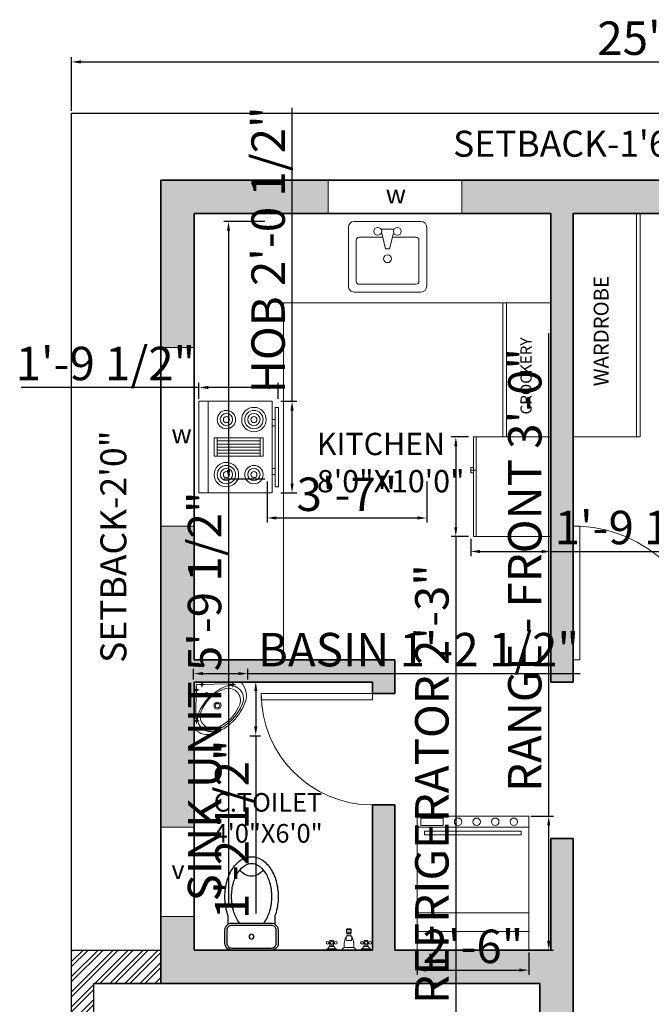
# Model space of a CAD drawing. Units: inches. Extents: x 3488 to 4319, y 780 to 1756.
# Tile 4 of 8: x 3509 to 3679, y 1491 to 1756. Entities that reach past the tile are written whole.
import ezdxf

# ---------------------------------------------------------------- set-up
doc = ezdxf.new("R2010")
doc.units = ezdxf.units.IN
for name, color, linetype, lineweight in [('A-ANNO-IDEN', 7, 'Continuous', 13), ('A-ANNO-TEXT', 7, 'Continuous', 18), ('A-AREA-IDEN', 7, 'Continuous', 18), ('A-DOOR', 4, 'Continuous', 18), ('A-EQPM', 8, 'Continuous', 18), ('A-FLOR-CASE', 32, 'Continuous', 18), ('A-WALL', 7, 'Continuous', 35), ('A-WALL-PATT', 252, 'Continuous', 13), ('C-PROP', 7, 'Continuous', 25), ('DIM', 9, 'Continuous', 18), ('L-FENC', 7, 'Continuous', 30), ('L-FENC-PATT', 251, 'Continuous', 13), ('window', 130, 'Continuous', 18), ('Сантехника', 9, 'Continuous', 18)]:
    doc.layers.add(name, color=color, linetype=linetype, lineweight=lineweight)
doc.layers.add('SANTEH', color=7, linetype='Continuous')
doc.styles.add('ATT', font='romans.shx')
doc.styles.get("Standard").update_dxf_attribs({"font": 'arial.ttf'})
doc.dimstyles.new('ISO-25', dxfattribs={"dimtxt": 9, "dimasz": 2.5, "dimexe": 1.25, "dimexo": 0.625, "dimtad": 1, "dimdec": 1, "dimlunit": 3, "dimtxsty": 'Standard', "dimcen": 2.5, "dimclrd": 1, "dimclre": 1, "dimclrt": 1, "dimadec": 0, "dimazin": 0, "dimtfac": 1, "dimtdec": 1, "dimtmove": 0, "dimatfit": 3, "dimfxl": 1, "dimarcsym": 0})

# ---------------------------------------------------------------- blocks, each defined once
blk = doc.blocks.new('*U3')
for p, q in [((0, 0), (0, -6)), ((36, 0), (36, -6))]:
    blk.add_line(p, q)
blk.add_lwpolyline([(0, 0), (0, 36), (1.75, 36), (1.75, 0)], close=True)
blk.add_arc((0, 0), 36, 0, 90)
blk = doc.blocks.new('*U4')
for p, q in [((-30, 0), (-30, -6)), ((0, 0), (0, -6))]:
    blk.add_line(p, q)
blk.add_lwpolyline([(0, 0), (0, 30), (-1.75, 30), (-1.75, 0)], close=True)
blk.add_arc((0, 0), 30, 90, 180)
blk = doc.blocks.new('*D5')
at = {"layer": 'Defpoints', "color": 0, "transparency": 16777216}
for p in [(3822.99, 1744.35), (3522.99, 1730.55), (3822.99, 1730.55)]:
    blk.add_point(p, dxfattribs=at)
at = {"layer": 'DIM', "color": 0, "lineweight": -2, "transparency": 16777216}
for p, q in [((3522.99, 1731.18), (3522.99, 1745.6)), ((3822.99, 1731.18), (3822.99, 1745.6)), ((3525.49, 1744.35), (3820.49, 1744.35))]:
    blk.add_line(p, q, dxfattribs=at)
at = {"layer": 'DIM', "color": 0, "transparency": 16777216}
for points in [[(3525.49, 1744.77), (3525.49, 1743.94), (3522.99, 1744.35)], [(3820.49, 1744.77), (3820.49, 1743.94), (3822.99, 1744.35)]]:
    blk.add_solid(points, dxfattribs=at)
at = {"layer": 'DIM', "color": 0, "transparency": 16777216, "insert": (3672.99, 1749.57), "char_height": 9, "attachment_point": 5}
blk.add_mtext("25'", dxfattribs=at)
blk = doc.blocks.new('s_11')
at = {"color": 0}
for p, q in [((-2.8, 5.7), (-3.1, 302.9)), ((-2.8, 5.7), (-3.1, 302.9)), ((11.5, 234), (11.4, 270.2)), ((-6.7, 252.1), (29.6, 252.1)), ((10.9, 19.3), (7.9, 238.3)), ((11.7, 31.1), (11.6, 67.3)), ((-6.5, 49.2), (29.8, 49.2)), ((237.1, 9.4), (18, 12.2)), ((29.8, 13), (66, 13)), ((47.9, -5.2), (47.9, 31.1)), ((232.7, 13), (268.9, 13)), ((250.8, -5.2), (250.8, 31.1)), ((301.6, -1.5), (4.5, -1.5)), ((301.6, -1.5), (4.5, -1.5))]:
    blk.add_line(p, q, dxfattribs=at)
at = {"color": 0, "extrusion": (0, 0, -1)}
for centre, major_axis, start_param, end_param in [((84.1, 218.8), (-87.2, 87.1), 0.025883, 1.117399), ((84.1, 218.8), (-87.2, 87.1), 0.025883, 1.117399), ((105.4, 236.4), (-61.5, 61.5), -1.180146, 1.180146), ((14.2, 15.4), (-239.5, 239.2), 1.117399, 2.024193), ((14.2, 15.4), (-239.5, 239.2), 1.117399, 2.024193), ((4.2, 302.9), (-5.13, 5.12), -0.785398, 0.025884), ((4.2, 302.9), (-5.13, 5.12), -0.785398, 0.025884), ((11.5, 252.1), (-5.13, 5.12), 3.141593, 9.424778), ((116.1, 223.2), (-56.4, 56.4), -1.140724, 1.140724), ((13.2, 14.4), (-231.7, 231.5), 1.180146, 1.961447), ((54, 55.3), (-183.1, 183), 1.140724, 2.000869), ((327.3, 328.9), (-231.7, 231.5), 4.321738, 5.10304), ((283.9, 285.4), (-183.1, 183), 4.282316, 5.142462), ((150.8, 152.2), (-16.4, 16.4), 3.141593, 9.424778), ((150.8, 152.2), (-10.3, 10.2), 3.141593, 9.424778), ((221.8, 117.6), (-56.4, 56.4), 2.000869, 4.282316), ((235, 106.9), (-61.5, 61.5), 1.961447, 4.321738), ((79.1, 80.4), (-8.98, 8.97), 3.141593, 9.424778), ((217.5, 85.5), (-87.2, 87.1), 2.024193, 3.11571), ((217.5, 85.5), (-87.2, 87.1), 2.024193, 3.11571), ((4.5, 5.7), (-5.13, 5.12), 3.926991, 5.497787), ((4.5, 5.7), (-5.13, 5.12), 3.926991, 5.497787), ((11.7, 49.2), (-5.13, 5.12), 3.141593, 9.424778), ((18.1, 19.4), (-5.13, 5.12), 3.939487, 5.485291), ((47.9, 13), (-5.13, 5.12), 3.141593, 9.424778), ((250.8, 13), (-5.13, 5.12), 3.141593, 9.424778), ((301.6, 5.7), (-5.13, 5.12), 3.115708, 3.926991), ((301.6, 5.7), (-5.13, 5.12), 3.115708, 3.926991)]:
    blk.add_ellipse(centre, major_axis=major_axis, ratio=0.999043, start_param=start_param, end_param=end_param, dxfattribs=at)
blk = doc.blocks.new('K10-44')
at = {"layer": 'SANTEH'}
for points in [[(-182, 222.6, 0.020439), (-174, 197.6), (-174, 134.8, 0.262987), (-198.2, 92), (-198.2, -8, 0.414214), (-148.2, -58), (151.8, -58, 0.414214), (201.8, -8), (201.8, 92, 0.262987), (177.6, 134.8), (177.6, 197.6, 0.020439), (185.6, 222.6, 0.067459), (201.8, 342, 0.067459), (185.6, 461.3, 0.079812), (143.2, 554.1, 0.107118), (73.7, 621.5, 0.139889), (1.8, 642, 0.139889), (-70.1, 621.5, 0.107118), (-139.6, 554.1, 0.079812), (-182, 461.3, 0.067459), (-198.2, 342, 0.067459)], [(-148.2, 127), (151.8, 127, -0.414214), (186.8, 92), (186.8, -8, -0.414214), (151.8, -43), (-148.2, -43, -0.414214), (-183.2, -8), (-183.2, 92, -0.414214)]]:
    blk.add_lwpolyline(points, format="xyb", close=True, dxfattribs=at)
for points in [[(89.9, 142, 0.027307), (101.6, 157.6, 0.079812), (137.4, 235.9, 0.067459), (151.8, 342, 0.067459), (137.4, 448, 0.079812), (101.6, 526.4, 0.107118), (47.3, 579, 0.139889), (1.8, 592, 0.139889), (-43.7, 579, 0.107118), (-98, 526.4, 0.079812), (-133.8, 448, 0.067459), (-148.2, 342, 0.067459), (-133.8, 235.9, 0.079812), (-98, 157.6, 0.027307), (-86.4, 142, 0.139889)], [(-174, 134.8, -0.136371), (-148.2, 142), (151.8, 142, -0.136371), (177.6, 134.8)]]:
    blk.add_lwpolyline(points, format="xyb", dxfattribs=at)
blk.add_circle((1.8, 42), 18.3, dxfattribs=at)
blk.add_arc((1.8, 601.6), 105.3, 213.89944, 326.10056, dxfattribs=at)
blk = doc.blocks.new('Faucet - Bathroom front')
for p, q in [((-0.5, 4.25), (0.5, 4.25)), ((0.5, 3.75), (-0.5, 3.75)), ((-0.5, 3), (0.5, 3)), ((-0.25, 3), (-0.25, 3.5)), ((0.25, 3.5), (0.25, 3)), ((-5, 0), (-2.25, 0)), ((-4.5087, 0.25), (-2.7408, 0.25)), ((-4, 1.625), (-4.25, 1.625)), ((-4, 1.375), (-4.25, 1.375)), ((-3.1442, 0.75), (-4.0979, 0.75)), ((-3.25, 1.625), (-3, 1.625)), ((-3.25, 1.375), (-3, 1.375)), ((-1.5, 0), (1.5, 0)), ((-1, 0.5), (1, 0.5)), ((0.5, 2), (-0.5, 2)), ((2.25, 0), (5, 0)), ((2.7413, 0.25), (4.5092, 0.25)), ((3.25, 1.625), (3, 1.625)), ((3.25, 1.375), (3, 1.375)), ((4.1058, 0.75), (3.1521, 0.75)), ((4, 1.625), (4.25, 1.625)), ((4, 1.375), (4.25, 1.375))]:
    blk.add_line(p, q)
for points in [[(-0.5, 3.75), (-0.5, 4.25)], [(-0.25, 4.5), (0.25, 4.5)], [(0.5, 4.25), (0.5, 3.75)], [(0.25, 3.5), (-0.25, 3.5)]]:
    blk.add_lwpolyline(points)
for points in [[(-4, 1), (-4, 2), (-3.25, 2), (-3.25, 1)], [(3.25, 1), (3.25, 2), (4, 2), (4, 1)]]:
    blk.add_lwpolyline(points, close=True)
for centre in [(-4.5, 1.5), (-3.625, 1.5), (-2.75, 1.5), (2.75, 1.5), (3.625, 1.5), (4.5, 1.5)]:
    blk.add_circle(centre, 0.2795)
for centre, radius, start, end in [((-0.2575, 4.2575), 0.2426, 88.22243, 181.7776), ((0.2575, 4.2575), 0.2426, 358.2224, 91.77757), ((3, 1), 4.0311, 150.2551, 187.125), ((0.6413, 2.5), 1.246, 156.3417, 203.6583), ((-0.2575, 3.7425), 0.2426, 178.2224, 271.7776), ((0.2575, 3.7425), 0.2426, 268.2224, 1.777565), ((-3, 1), 4.0311, 352.875, 29.74488), ((-0.6413, 2.5), 1.246, 336.3417, 23.65835), ((-5.375, 1.375), 1.4252, 285.2551, 344.7449), ((-1.875, 1.375), 1.4252, 195.2551, 254.7449), ((-0.7962, -0.2038), 0.7327, 106.1502, 163.8498), ((0.7962, -0.2038), 0.7327, 16.1502, 73.84979), ((1.875, 1.375), 1.4252, 285.2551, 344.7449), ((5.375, 1.375), 1.4252, 195.2551, 254.7449)]:
    blk.add_arc(centre, radius, start, end)
blk = doc.blocks.new('Range-Oven - 30 in top')
for p, q in [((0, -3), (30, -3)), ((12, -6), (18, -6)), ((13, -20), (13, -6)), ((14, -6), (14, -20)), ((15, -20), (15, -6)), ((16, -6), (16, -20)), ((17, -20), (17, -6)), ((18, -20), (12, -20)), ((6, -24), (6, -25)), ((8, -25), (8, -24)), ((22, -25), (22, -24)), ((24, -24), (24, -25))]:
    blk.add_line(p, q)
for points in [[(0, -24), (0, 0), (30, 0), (30, -24)], [(12, -21), (12, -5), (18, -5), (18, -21)], [(2, -26), (2, -25), (28, -25), (28, -26)]]:
    blk.add_lwpolyline(points, close=True)
for centre, radius in [((6, -9), 4), ((6, -9), 3), ((24, -9), 3), ((6, -9), 2), ((6, -9), 1), ((24, -9), 2), ((24, -9), 1), ((6, -18), 3), ((6, -18), 2), ((24, -18), 4), ((24, -18), 3), ((24, -18), 2), ((6, -18), 1), ((24, -18), 1)]:
    blk.add_circle(centre, radius)
blk = doc.blocks.new('Range-Oven - 30 in front')
for p, q in [((0, 33.00005), (30, 33.00005)), ((30, 10), (0, 10)), ((0, 5), (30, 5))]:
    blk.add_line(p, q)
for points in [[(0, 0), (0, 36.00005), (30, 36.00005), (30, 0)], [(1, 33.50005), (1, 35.50005), (7, 35.50005), (7, 33.50005)], [(2, 31.00005), (2, 32.00005), (28, 32.00005), (28, 31.00005)]]:
    blk.add_lwpolyline(points, close=True)
for centre in [(11, 34.50005), (16, 34.50005), (21, 34.50005), (26, 34.50005)]:
    blk.add_circle(centre, 1)
blk = doc.blocks.new('Refrigerator-2 door - 36 in top')
for p, q in [((0, -26.999999), (36, -26.999999)), ((11, -27.999999), (11, -28.999999)), ((12, -26.999999), (12, -28.999999)), ((13, -28.999999), (13, -27.999999)), ((11, -28.999999), (13, -28.999999))]:
    blk.add_line(p, q)
blk.add_lwpolyline([(0, -27.999999), (0, 0), (36, 0), (36, -27.999999)], close=True)
blk = doc.blocks.new('15PLAV06')
at = {"color": 0, "linetype": 'ByBlock'}
for p, q in [((0, 8.5), (0, -8.5)), ((16.5, 10), (1.5, 10)), ((4.75, 8), (15.25, 8)), ((18, -8.5), (18, 8.5)), ((4, 1.25), (4, 7.25)), ((16, 7.25), (16, -7.25)), ((2, -1.5), (2, 1.5)), ((7, 0.5), (3, 1.5)), ((7, -0.5), (7, 0.5)), ((3, -1.5), (7, -0.5)), ((4, -7.25), (4, -1.25)), ((1.5, -10), (16.5, -10)), ((15.25, -8), (4.75, -8))]:
    blk.add_line(p, q, dxfattribs=at)
for centre in [(2.5, 2.5), (9.5, 0), (2.5, -2.5)]:
    blk.add_circle(centre, 1, dxfattribs=at)
for centre, radius, start, end in [((1.5, 8.5), 1.5, 90, 180), ((4.75, 7.25), 0.75, 90, 180), ((15.25, 7.25), 0.75, 0, 90), ((16.5, 8.5), 1.5, 0, 90), ((4.75, -7.25), 0.75, 180, 270), ((15.25, -7.25), 0.75, 270, 0), ((1.5, -8.5), 1.5, 180, 270), ((16.5, -8.5), 1.5, 270, 0)]:
    blk.add_arc(centre, radius, start, end, dxfattribs=at)
at = {"color": 0, "linetype": 'ByBlock', "style": 'ATT'}
for tag, p, flags in [('ITEM', (0, -20), 3), ('ROOM_NUMBER', (0, -29), 1)]:
    blk.add_attdef(tag, p, '', height=6, dxfattribs=dict(at, flags=flags))
blk = doc.blocks.new('*D84')
at = {"layer": 'Defpoints', "color": 0, "transparency": 16777216}
for p in [(3570.37, 1579.88), (3555.83, 1577.7), (3570.37, 1577.7)]:
    blk.add_point(p, dxfattribs=at)
at = {"layer": 'DIM', "color": 1, "lineweight": -2, "transparency": 16777216}
for p, q in [((3555.83, 1578.33), (3555.83, 1581.13)), ((3570.37, 1578.33), (3570.37, 1581.13)), ((3558.33, 1579.88), (3567.87, 1579.88)), ((3570.37, 1579.88), (3659.84, 1579.88))]:
    blk.add_line(p, q, dxfattribs=at)
at = {"layer": 'DIM', "color": 1, "transparency": 16777216}
for points in [[(3558.33, 1580.3), (3558.33, 1579.46), (3555.83, 1579.88)], [(3567.87, 1580.3), (3567.87, 1579.46), (3570.37, 1579.88)]]:
    blk.add_solid(points, dxfattribs=at)
at = {"layer": 'DIM', "color": 1, "transparency": 16777216, "insert": (3616.35, 1585.16), "char_height": 9, "attachment_point": 5}
blk.add_mtext('BASIN 1\'-2 1/2"', dxfattribs=at)
blk = doc.blocks.new('*D85')
at = {"layer": 'Defpoints', "color": 0, "transparency": 16777216}
for p in [(3570.37, 1577.7), (3570.37, 1563.17), (3572.55, 1563.17)]:
    blk.add_point(p, dxfattribs=at)
at = {"layer": 'DIM', "color": 1, "lineweight": -2, "transparency": 16777216}
for p, q in [((3570.99, 1577.7), (3573.8, 1577.7)), ((3572.55, 1575.2), (3572.55, 1565.67)), ((3570.99, 1563.17), (3573.8, 1563.17)), ((3572.55, 1563.17), (3572.55, 1515.37))]:
    blk.add_line(p, q, dxfattribs=at)
at = {"layer": 'DIM', "color": 1, "transparency": 16777216}
for points in [[(3572.13, 1575.2), (3572.96, 1575.2), (3572.55, 1577.7)], [(3572.13, 1565.67), (3572.96, 1565.67), (3572.55, 1563.17)]]:
    blk.add_solid(points, dxfattribs=at)
at = {"layer": 'DIM', "color": 1, "transparency": 16777216, "insert": (3567.27, 1538.02), "char_height": 9, "attachment_point": 5, "rotation": 90}
blk.add_mtext('1\'-2 1/2"', dxfattribs=at)
blk = doc.blocks.new('*D86')
at = {"layer": 'Defpoints', "color": 0, "transparency": 16777216}
for p in [(3578.62, 1653.11), (3582.32, 1653.11), (3578.62, 1628.45)]:
    blk.add_point(p, dxfattribs=at)
at = {"layer": 'DIM', "color": 1, "lineweight": -2, "transparency": 16777216}
for p, q in [((3582.32, 1653.11), (3582.32, 1732.01)), ((3579.25, 1653.11), (3583.57, 1653.11)), ((3582.32, 1630.95), (3582.32, 1650.61)), ((3579.25, 1628.45), (3583.57, 1628.45))]:
    blk.add_line(p, q, dxfattribs=at)
at = {"layer": 'DIM', "color": 1, "transparency": 16777216}
for points in [[(3581.9, 1650.61), (3582.74, 1650.61), (3582.32, 1653.11)], [(3581.9, 1630.95), (3582.74, 1630.95), (3582.32, 1628.45)]]:
    blk.add_solid(points, dxfattribs=at)
at = {"layer": 'DIM', "color": 1, "transparency": 16777216, "insert": (3577.04, 1693.81), "char_height": 9, "attachment_point": 5, "rotation": 90}
blk.add_mtext('HOB 2\'-0 1/2"', dxfattribs=at)
blk = doc.blocks.new('*D87')
at = {"layer": 'Defpoints', "color": 0, "transparency": 16777216}
for p in [(3557.25, 1656.81), (3557.25, 1653.11), (3578.62, 1653.11)]:
    blk.add_point(p, dxfattribs=at)
at = {"layer": 'DIM', "color": 1, "lineweight": -2, "transparency": 16777216}
for p, q in [((3557.25, 1653.74), (3557.25, 1658.06)), ((3578.62, 1653.74), (3578.62, 1658.06)), ((3557.25, 1656.81), (3509.45, 1656.81)), ((3576.12, 1656.81), (3559.75, 1656.81))]:
    blk.add_line(p, q, dxfattribs=at)
at = {"layer": 'DIM', "color": 1, "transparency": 16777216}
for points in [[(3559.75, 1657.23), (3559.75, 1656.39), (3557.25, 1656.81)], [(3576.12, 1657.23), (3576.12, 1656.39), (3578.62, 1656.81)]]:
    blk.add_solid(points, dxfattribs=at)
at = {"layer": 'DIM', "color": 1, "transparency": 16777216, "insert": (3532.1, 1662.09), "char_height": 9, "attachment_point": 5}
blk.add_mtext('1\'-9 1/2"', dxfattribs=at)
blk = doc.blocks.new('*D88')
at = {"layer": 'Defpoints', "color": 0, "transparency": 16777216}
for p in [(3645.99, 1541.55), (3651.39, 1541.55), (3645.99, 1505.55)]:
    blk.add_point(p, dxfattribs=at)
at = {"layer": 'DIM', "color": 1, "lineweight": -2, "transparency": 16777216}
for p, q in [((3651.39, 1541.55), (3651.39, 1671.44)), ((3646.61, 1541.55), (3652.64, 1541.55)), ((3651.39, 1508.05), (3651.39, 1539.05)), ((3646.61, 1505.55), (3652.64, 1505.55))]:
    blk.add_line(p, q, dxfattribs=at)
at = {"layer": 'DIM', "color": 1, "transparency": 16777216}
for points in [[(3650.97, 1539.05), (3651.81, 1539.05), (3651.39, 1541.55)], [(3650.97, 1508.05), (3651.81, 1508.05), (3651.39, 1505.55)]]:
    blk.add_solid(points, dxfattribs=at)
at = {"layer": 'DIM', "color": 1, "transparency": 16777216, "insert": (3646.1, 1607.75), "char_height": 9, "attachment_point": 5, "rotation": 90}
blk.add_mtext('RANGE - FRONT 3\'-0"', dxfattribs=at)
blk = doc.blocks.new('*D89')
at = {"layer": 'Defpoints', "color": 0, "transparency": 16777216}
for p in [(3615.99, 1505.55), (3645.99, 1505.55), (3645.99, 1500.15)]:
    blk.add_point(p, dxfattribs=at)
at = {"layer": 'DIM', "color": 1, "lineweight": -2, "transparency": 16777216}
for p, q in [((3615.99, 1504.93), (3615.99, 1498.9)), ((3645.99, 1504.93), (3645.99, 1498.9)), ((3618.49, 1500.15), (3643.49, 1500.15))]:
    blk.add_line(p, q, dxfattribs=at)
at = {"layer": 'DIM', "color": 1, "transparency": 16777216}
for points in [[(3618.49, 1500.57), (3618.49, 1499.74), (3615.99, 1500.15)], [(3643.49, 1500.57), (3643.49, 1499.74), (3645.99, 1500.15)]]:
    blk.add_solid(points, dxfattribs=at)
at = {"layer": 'DIM', "color": 1, "transparency": 16777216, "insert": (3630.99, 1505.37), "char_height": 9, "attachment_point": 5}
blk.add_mtext('2\'-6"', dxfattribs=at)
blk = doc.blocks.new('*D90')
at = {"layer": 'Defpoints', "color": 0, "transparency": 16777216}
for p in [(3630.4, 1643.52), (3626.38, 1616.73), (3630.4, 1616.73)]:
    blk.add_point(p, dxfattribs=at)
at = {"layer": 'DIM', "color": 1, "lineweight": -2, "transparency": 16777216}
for p, q in [((3629.78, 1643.52), (3625.13, 1643.52)), ((3626.38, 1641.02), (3626.38, 1619.23)), ((3629.78, 1616.73), (3625.13, 1616.73)), ((3626.38, 1616.73), (3626.38, 1486.14))]:
    blk.add_line(p, q, dxfattribs=at)
at = {"layer": 'DIM', "color": 1, "transparency": 16777216}
for points in [[(3625.97, 1641.02), (3626.8, 1641.02), (3626.38, 1643.52)], [(3625.97, 1619.23), (3626.8, 1619.23), (3626.38, 1616.73)]]:
    blk.add_solid(points, dxfattribs=at)
at = {"layer": 'DIM', "color": 1, "transparency": 16777216, "insert": (3621.1, 1550.18), "char_height": 9, "attachment_point": 5, "rotation": 90}
blk.add_mtext('REFRIGERATOR 2\'-3"', dxfattribs=at)
blk = doc.blocks.new('*D91')
at = {"layer": 'Defpoints', "color": 0, "transparency": 16777216}
for p in [(3630.4, 1616.73), (3651.99, 1616.73), (3651.99, 1612.71)]:
    blk.add_point(p, dxfattribs=at)
at = {"layer": 'DIM', "color": 1, "lineweight": -2, "transparency": 16777216}
for p, q in [((3630.4, 1616.1), (3630.4, 1611.46)), ((3651.99, 1616.1), (3651.99, 1611.46)), ((3632.9, 1612.71), (3649.49, 1612.71)), ((3651.99, 1612.71), (3699.79, 1612.71))]:
    blk.add_line(p, q, dxfattribs=at)
at = {"layer": 'DIM', "color": 1, "transparency": 16777216}
for points in [[(3632.9, 1613.13), (3632.9, 1612.29), (3630.4, 1612.71)], [(3649.49, 1613.13), (3649.49, 1612.29), (3651.99, 1612.71)]]:
    blk.add_solid(points, dxfattribs=at)
at = {"layer": 'DIM', "color": 1, "transparency": 16777216, "insert": (3677.14, 1617.99), "char_height": 9, "attachment_point": 5}
blk.add_mtext('1\'-9 1/2"', dxfattribs=at)
blk = doc.blocks.new('*D92')
at = {"layer": 'Defpoints', "color": 0, "transparency": 16777216}
for p in [(3575.62, 1701.45), (3565.22, 1632.12), (3575.62, 1632.12)]:
    blk.add_point(p, dxfattribs=at)
at = {"layer": 'DIM', "color": 1, "lineweight": -2, "transparency": 16777216}
for p, q in [((3575, 1701.45), (3563.97, 1701.45)), ((3565.22, 1698.95), (3565.22, 1634.62)), ((3575, 1632.12), (3563.97, 1632.12)), ((3565.22, 1632.12), (3565.22, 1517.85))]:
    blk.add_line(p, q, dxfattribs=at)
at = {"layer": 'DIM', "color": 1, "transparency": 16777216}
for points in [[(3564.8, 1698.95), (3565.64, 1698.95), (3565.22, 1701.45)], [(3564.8, 1634.62), (3565.64, 1634.62), (3565.22, 1632.12)]]:
    blk.add_solid(points, dxfattribs=at)
at = {"layer": 'DIM', "color": 1, "transparency": 16777216, "insert": (3559.94, 1573.74), "char_height": 9, "attachment_point": 5, "rotation": 90}
blk.add_mtext('SINK UNIT 5\'-9 1/2"', dxfattribs=at)
blk = doc.blocks.new('*D93')
at = {"layer": 'Defpoints', "color": 0, "transparency": 16777216}
for p in [(3575.62, 1632.12), (3618.56, 1632.12), (3618.56, 1621.72)]:
    blk.add_point(p, dxfattribs=at)
at = {"layer": 'DIM', "color": 1, "lineweight": -2, "transparency": 16777216}
for p, q in [((3575.62, 1631.5), (3575.62, 1620.47)), ((3618.56, 1631.5), (3618.56, 1620.47)), ((3578.12, 1621.72), (3616.06, 1621.72))]:
    blk.add_line(p, q, dxfattribs=at)
at = {"layer": 'DIM', "color": 1, "transparency": 16777216}
for points in [[(3578.12, 1622.14), (3578.12, 1621.3), (3575.62, 1621.72)], [(3616.06, 1622.14), (3616.06, 1621.3), (3618.56, 1621.72)]]:
    blk.add_solid(points, dxfattribs=at)
at = {"layer": 'DIM', "color": 1, "transparency": 16777216, "insert": (3597.09, 1626.94), "char_height": 9, "attachment_point": 5}
blk.add_mtext('3\'-7"', dxfattribs=at)

msp = doc.modelspace()

# ---------------------------------------------------------------- hatches: boundary and pattern name
at = {"layer": 'A-WALL-PATT', "transparency": 33554687}
h = msp.add_hatch(color=256, dxfattribs=at)
h.dxf.hatch_style = 1
h.paths.add_polyline_path([(3657.99, 1505.55), (3657.99, 1535.55), (3651.99, 1535.55), (3651.99, 1505.55), (3609.99, 1505.55), (3609.99, 1544.55), (3603.99, 1544.55), (3603.99, 1505.55), (3555.99, 1505.55), (3555.99, 1514.55), (3546.99, 1514.55), (3546.99, 1496.55), (3648.99, 1496.55), (3648.99, 1352.55), (3663.99, 1352.55), (3663.99, 1361.55), (3657.99, 1361.55)])
h.paths.add_polyline_path([(3722.99, 1361.55), (3719, 1361.55), (3703.99, 1361.55), (3703.99, 1352.55), (3722.99, 1352.55)])
h.paths.add_polyline_path([(3798.99, 1397.55), (3789.99, 1397.55), (3789.99, 1361.95), (3789.99, 1361.55), (3770.99, 1361.55), (3770.99, 1352.55), (3798.99, 1352.55)])
h.paths.add_polyline_path([(3798.99, 1547.58), (3789.99, 1547.58), (3789.99, 1463.55), (3798.99, 1463.55)])
h.paths.add_polyline_path([(3798.99, 1613.55), (3789.99, 1613.55), (3789.99, 1583.55), (3693.99, 1583.55), (3693.99, 1577.55), (3789.99, 1577.55), (3789.99, 1571.58), (3798.99, 1571.58)])
h.paths.add_polyline_path([(3798.99, 1712.55), (3717.99, 1712.55), (3717.99, 1703.55), (3789.99, 1703.55), (3789.99, 1673.55), (3798.99, 1673.55)])
h.paths.add_polyline_path([(3681.99, 1712.55), (3627.99, 1712.55), (3627.99, 1703.55), (3651.99, 1703.55), (3651.99, 1577.55), (3657.99, 1577.55), (3657.99, 1703.55), (3681.99, 1703.55)])
h.paths.add_polyline_path([(3591.99, 1712.55), (3546.99, 1712.55), (3546.99, 1667.55), (3555.99, 1667.55), (3555.99, 1703.55), (3591.99, 1703.55)])
edge = h.paths.add_edge_path()
edge.add_line((3555.99, 1619.55), (3546.99, 1619.55))
edge.add_line((3546.99, 1619.55), (3546.99, 1538.55))
edge.add_line((3546.99, 1538.55), (3555.99, 1538.55))
edge.add_line((3555.99, 1538.55), (3555.99, 1565.03))
edge.add_ellipse((3556.27, 1565.11), major_axis=(0.21, 0.21), ratio=0.999043, start_angle=135, end_angle=151.1563, ccw=False)
edge.add_line((3555.98, 1565.08), (3555.99, 1577.26))
edge.add_line((3555.99, 1577.26), (3555.99, 1577.55))
edge.add_line((3555.99, 1577.55), (3603.99, 1577.55))
edge.add_line((3603.99, 1577.55), (3603.99, 1574.55))
edge.add_line((3603.99, 1574.55), (3609.99, 1574.55))
edge.add_line((3609.99, 1574.55), (3609.99, 1583.55))
edge.add_line((3609.99, 1583.55), (3555.99, 1583.55))
edge.add_line((3555.99, 1583.55), (3555.99, 1619.55))
at = {"layer": 'L-FENC-PATT', "transparency": 33554687}
h = msp.add_hatch(dxfattribs=at)
h.set_pattern_fill('ANSI32', color=256, scale=0.3)
h.paths.add_polyline_path([(3546.99, 1505.55), (3522.99, 1505.55), (3522.99, 1310.55), (3546.99, 1310.55), (3546.99, 1316.55), (3528.99, 1316.55), (3528.99, 1496.55), (3546.99, 1496.55)])
h.paths.add_polyline_path([(3756.99, 1316.55), (3642.99, 1316.55), (3642.99, 1310.55), (3756.99, 1310.55)])
h.paths.add_polyline_path([(3822.99, 1316.55), (3792.99, 1316.55), (3792.99, 1310.55), (3822.99, 1310.55)])

# ---------------------------------------------------------------- linework, layer by layer
at = {"layer": 'A-FLOR-CASE'}
for p, q in [((3674.99, 1703.55), (3674.99, 1643.55)), ((3675.99, 1703.55), (3675.99, 1643.55)), ((3579.99, 1679.55), (3651.99, 1679.55)), ((3579.99, 1583.55), (3579.99, 1679.55)), ((3638.99, 1679.55), (3638.99, 1643.52)), ((3639.99, 1679.55), (3639.99, 1643.52)), ((3657.99, 1643.55), (3675.99, 1643.55))]:
    msp.add_line(p, q, dxfattribs=at)
at = {"layer": 'A-WALL'}
for p, q in [((3546.99, 1712.55), (3798.99, 1712.55)), ((3546.99, 1496.55), (3546.99, 1712.55)), ((3555.99, 1703.55), (3651.99, 1703.55)), ((3555.99, 1583.55), (3555.99, 1703.55)), ((3651.99, 1703.55), (3651.99, 1577.55)), ((3657.99, 1703.55), (3657.99, 1577.55)), ((3657.99, 1703.55), (3789.99, 1703.55)), ((3555.99, 1583.55), (3609.99, 1583.55)), ((3609.99, 1574.55), (3609.99, 1583.55)), ((3555.99, 1505.55), (3555.99, 1577.55)), ((3555.99, 1577.55), (3603.99, 1577.55)), ((3603.99, 1574.55), (3603.99, 1577.55)), ((3651.99, 1577.55), (3657.99, 1577.55)), ((3603.99, 1574.55), (3609.99, 1574.55)), ((3603.99, 1505.55), (3603.99, 1544.55)), ((3603.99, 1544.55), (3609.99, 1544.55)), ((3609.99, 1505.55), (3609.99, 1544.55)), ((3651.99, 1535.55), (3657.99, 1535.55)), ((3651.99, 1535.55), (3651.99, 1505.55)), ((3657.99, 1535.55), (3657.99, 1505.55)), ((3555.99, 1505.55), (3603.99, 1505.55)), ((3609.99, 1505.55), (3651.99, 1505.55)), ((3657.99, 1505.55), (3657.99, 1361.55)), ((3528.99, 1496.55), (3648.99, 1496.55)), ((3648.99, 1496.55), (3648.99, 1352.55))]:
    msp.add_line(p, q, dxfattribs=at)
at = {"layer": 'C-PROP'}
for p, q in [((3522.99, 1730.55), (3822.99, 1730.55)), ((3522.99, 1310.55), (3522.99, 1730.55))]:
    msp.add_line(p, q, dxfattribs=at)
at = {"layer": 'L-FENC'}
for p, q in [((3522.99, 1505.55), (3546.99, 1505.55)), ((3528.99, 1316.55), (3528.99, 1496.55))]:
    msp.add_line(p, q, dxfattribs=at)
at = {"layer": 'window'}
for p, q in [((3591.99, 1703.55), (3591.99, 1712.55)), ((3627.99, 1703.55), (3627.99, 1712.55)), ((3555.99, 1667.55), (3546.99, 1667.55)), ((3555.99, 1619.55), (3546.99, 1619.55)), ((3546.99, 1538.55), (3555.99, 1538.55)), ((3546.99, 1514.55), (3555.99, 1514.55))]:
    msp.add_line(p, q, dxfattribs=at)

# ---------------------------------------------------------------- block references
at = {"layer": 'A-DOOR'}
msp.add_blockref('*U3', (3657.99, 1583.55), dxfattribs=at)
at = {"layer": 'A-DOOR', "rotation": 90}
msp.add_blockref('*U4', (3603.99, 1574.55), dxfattribs=at)
at = {"layer": 'A-EQPM'}
for name, p, xscale, yscale, zscale, rotation in [('Range-Oven - 30 in top', (3557.25, 1628.45), 0.8221221388671134, 0.8221221388671134, 0.8221221388671134, 90), ('Refrigerator-2 door - 36 in top', (3651.99, 1643.52), 0.7443170329711898, 0.7443170329711898, 0.7443170329711898, 270)]:
    msp.add_blockref(name, p, dxfattribs=dict(at, xscale=xscale, yscale=yscale, zscale=zscale, rotation=rotation))
msp.add_blockref('Range-Oven - 30 in front', (3615.99, 1505.55), dxfattribs=at)
at = {"layer": 'Сантехника'}
for name, p, xscale, yscale, zscale, rotation in [('15PLAV06', (3608.01, 1701.45), 1.054623354967256, 1.054623354967256, 1.054623354967256, 270), ('s_11', (3556.1, 1577.49), -0.0408764858577606, 0.0408764858577606, 0.0408764858577606, 180)]:
    msp.add_blockref(name, p, dxfattribs=dict(at, xscale=xscale, yscale=yscale, zscale=zscale, rotation=rotation))
for name, p, xscale, yscale, zscale in [('K10-44', (3571.48, 1507.63), -0.0358529150226637, 0.0358529150226637, 0.0358529150226637), ('Faucet - Bathroom front', (3597.62, 1505.55), 1.274234813154425, 1.274234813154425, 1.274234813154425)]:
    msp.add_blockref(name, p, dxfattribs=dict(at, xscale=xscale, yscale=yscale, zscale=zscale))

# ---------------------------------------------------------------- texts
at = {"layer": 'A-ANNO-IDEN'}
for s, p in [('w', (3607.51, 1706.3)), ('w', (3549.85, 1641.84)), ('v', (3549.85, 1524.64))]:
    msp.add_text(s, height=5, dxfattribs=at).set_placement(p)
at = {"layer": 'A-ANNO-TEXT', "insert": (3625.66, 1725.86), "char_height": 7, "attachment_point": 1}
msp.add_mtext_dynamic_manual_height_columns('\\pxt7;{SETBACK-1\'6"}', width=83.4163, gutter_width=25, heights=[0], dxfattribs=at)
at = {"layer": 'A-ANNO-TEXT', "attachment_point": 1, "rotation": 90}
for s, insert, char_height in [('WARDROBE', (3663.48, 1657.14), 4), ('CROCKERY', (3643.78, 1649.56), 3), ('\\pxt7;{SETBACK-2\'0"}', (3530.74, 1582.77), 7)]:
    msp.add_mtext_dynamic_manual_height_columns(s, width=83.4163, gutter_width=25, heights=[0], dxfattribs=dict(at, insert=insert, char_height=char_height))
at = {"layer": 'A-AREA-IDEN', "attachment_point": 1}
for s, insert, char_height in [('KITCHEN\\P8\'0"X10\'0"', (3589, 1644.62), 6), ('C.TOILET\\P4\'0"X6\'0"', (3561.23, 1547.76), 5)]:
    msp.add_mtext_dynamic_manual_height_columns(s, width=83.4163, gutter_width=25, heights=[0], dxfattribs=dict(at, insert=insert, char_height=char_height))

# ---------------------------------------------------------------- dimensions: what is measured, and where the dimension line sits
at = {"layer": 'DIM'}
for base, p1, p2, override, picture, middle in [((3822.99, 1744.35), (3522.99, 1730.55), (3822.99, 1730.55), {"dimclrd": 0, "dimclre": 0, "dimclrt": 0}, '*D5', (3672.99, 1749.57)), ((3618.56, 1621.72), (3575.62, 1632.12), (3618.56, 1632.12), {"dimdec": 1, "dimlfac": 1, "dimrnd": 0, "dimzin": 1, "dimdsep": 46, "dimlunit": 4, "dimfrac": 2}, '*D93', (3597.09, 1626.94)), ((3651.99, 1612.71), (3630.4, 1616.73), (3651.99, 1616.73), {"dimdec": 1, "dimlfac": 1, "dimrnd": 0, "dimzin": 1, "dimdsep": 46, "dimlunit": 4, "dimfrac": 2}, '*D91', (3677.14, 1617.99)), ((3645.99, 1500.15), (3615.99, 1505.55), (3645.99, 1505.55), {"dimdec": 1, "dimlfac": 1, "dimrnd": 0, "dimzin": 1, "dimdsep": 46, "dimlunit": 4, "dimfrac": 2}, '*D89', (3630.99, 1505.37))]:
    dim = msp.add_linear_dim(base=base, p1=p1, p2=p2, dimstyle='ISO-25', override=override, dxfattribs=at)
    dim.commit()
    dim.dimension.update_dxf_attribs({"geometry": picture, "text_midpoint": middle})
for base, p1, p2, angle, text, picture, middle in [((3582.32, 1653.11), (3578.62, 1628.45), (3578.62, 1653.11), 90, 'HOB <>', '*D86', (3577.04, 1693.81)), ((3565.22, 1632.12), (3575.62, 1701.45), (3575.62, 1632.12), 270, 'SINK UNIT <>', '*D92', (3559.94, 1573.74)), ((3651.39, 1541.55), (3645.99, 1505.55), (3645.99, 1541.55), 90, 'RANGE - FRONT <>', '*D88', (3646.1, 1607.75)), ((3626.38, 1616.73), (3630.4, 1643.52), (3630.4, 1616.73), 270, 'REFRIGERATOR <>', '*D90', (3621.1, 1550.18))]:
    dim = msp.add_linear_dim(base=base, p1=p1, p2=p2, angle=angle, text=text, dimstyle='ISO-25', override={"dimdec": 1, "dimlfac": 1, "dimrnd": 0, "dimzin": 1, "dimdsep": 46, "dimlunit": 4, "dimfrac": 2}, dxfattribs=at)
    dim.commit()
    dim.dimension.update_dxf_attribs({"geometry": picture, "text_midpoint": middle})
for base, p1, p2, angle, picture, middle in [((3557.25, 1656.81), (3578.62, 1653.11), (3557.25, 1653.11), 180, '*D87', (3532.1, 1662.09)), ((3572.55, 1563.17), (3570.37, 1577.7), (3570.37, 1563.17), 270, '*D85', (3567.27, 1538.02))]:
    dim = msp.add_linear_dim(base=base, p1=p1, p2=p2, angle=angle, dimstyle='ISO-25', override={"dimdec": 1, "dimlfac": 1, "dimrnd": 0, "dimzin": 1, "dimdsep": 46, "dimlunit": 4, "dimfrac": 2}, dxfattribs=at)
    dim.commit()
    dim.dimension.update_dxf_attribs({"geometry": picture, "text_midpoint": middle})
dim = msp.add_linear_dim(base=(3570.37, 1579.88), p1=(3555.83, 1577.7), p2=(3570.37, 1577.7), text='BASIN <>', dimstyle='ISO-25', override={"dimdec": 1, "dimlfac": 1, "dimrnd": 0, "dimzin": 1, "dimdsep": 46, "dimlunit": 4, "dimfrac": 2}, dxfattribs=at)
dim.commit()
dim.dimension.update_dxf_attribs({"geometry": '*D84', "text_midpoint": (3616.35, 1585.16)})

doc.saveas('drawing.dxf')
